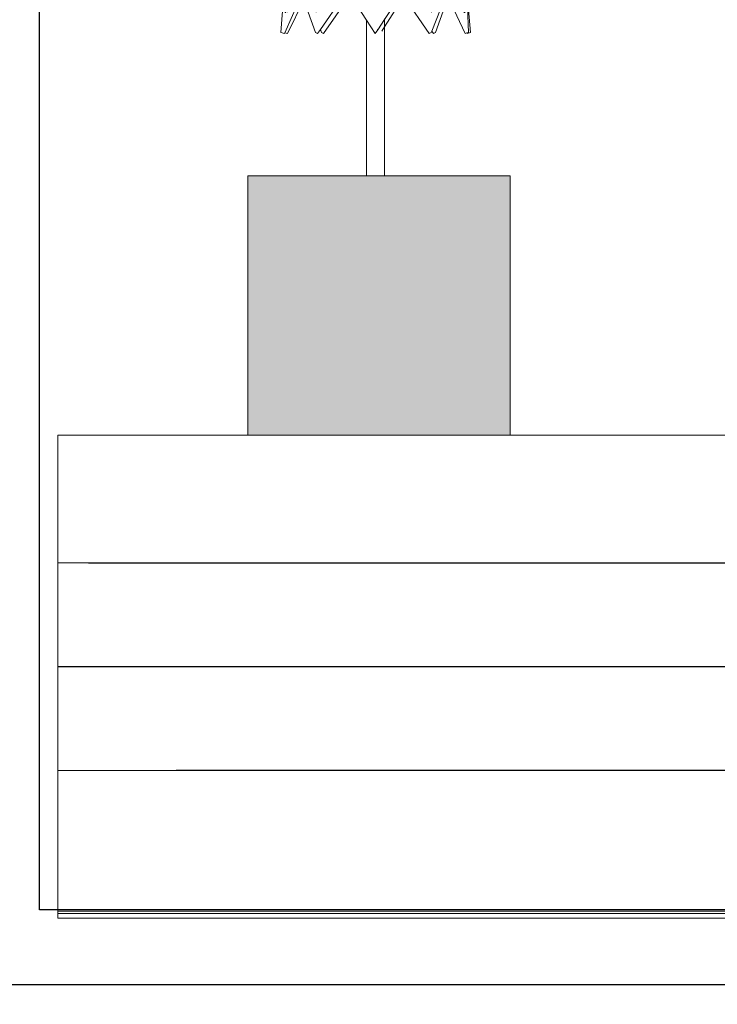
# Model space of a CAD drawing. Units: millimetres. Extents: x 7894 to 8038, y 6851 to 6951.
# Tile 3 of 49: x 7944.854 to 7949.503, y 6864.931 to 6871.489. Entities that reach past the tile are written whole.
import ezdxf

# ---------------------------------------------------------------- set-up
doc = ezdxf.new("R2010")
doc.units = ezdxf.units.MM
for name, color, linetype, lineweight in [('A-ANNO-DIMS', 2, 'Continuous', 18), ('A-FURN-ACCS', 8, 'Continuous', 13), ('A-FURN-BOOK', 8, 'Continuous', 13), ('A-FURN-CASE', 7, 'Continuous', 30)]:
    doc.layers.add(name, color=color, linetype=linetype, lineweight=lineweight)
doc.layers.add('A-FURN-ACCS-PATT', color=116, linetype='Continuous', lineweight=9, true_color=0x136734)
doc.styles.get("Standard").update_dxf_attribs({"font": 'arial.ttf'})
doc.dimstyles.new('ISO-25', dxfattribs={"dimtxt": 1, "dimasz": 1, "dimexe": 1.25, "dimexo": 0.625, "dimtad": 1, "dimdec": 0, "dimlunit": 4, "dimtxsty": 'Standard', "dimcen": 2.5, "dimclrt": 1, "dimadec": 0, "dimazin": 0, "dimtfac": 1, "dimtdec": 0, "dimtmove": 0, "dimatfit": 3, "dimfxl": 1, "dimarcsym": 0})

# ---------------------------------------------------------------- blocks, each defined once
blk = doc.blocks.new('DISPLAY-LEAF-FINIAL')
for p, q in [((2.4341, 3.4699), (2.4472, 3.4778)), ((2.4472, 3.4778), (2.4609, 3.4849)), ((2.4609, 3.4849), (2.475, 3.4911)), ((2.475, 3.4911), (2.4894, 3.4964)), ((2.4894, 3.4964), (2.5041, 3.5007)), ((2.5041, 3.5007), (2.5191, 3.5041)), ((2.5634, 3.479), (2.5605, 3.4646)), ((2.5649, 3.4937), (2.5634, 3.479)), ((2.565, 3.5085), (2.5649, 3.4937)), ((2.2094, 3.3343), (2.2756, 3.4413)), ((2.2756, 3.4413), (2.398, 3.4413)), ((2.398, 3.4413), (2.4094, 3.4516)), ((2.4094, 3.4516), (2.4214, 3.4612)), ((2.4214, 3.4612), (2.4341, 3.4699)), ((2.5358, 3.4113), (2.5266, 3.3997)), ((2.5438, 3.4237), (2.5358, 3.4113)), ((2.5507, 3.4368), (2.5438, 3.4237)), ((2.5562, 3.4504), (2.5507, 3.4368)), ((2.5605, 3.4646), (2.5562, 3.4504)), ((2.4932, 3.3709), (2.4804, 3.3635)), ((2.4804, 3.3635), (2.4804, 3.3164)), ((2.5053, 3.3794), (2.4932, 3.3709)), ((2.5164, 3.3891), (2.5053, 3.3794)), ((2.5266, 3.3997), (2.5164, 3.3891)), ((2.5489, 3.3378), (2.5584, 3.3473)), ((2.5584, 3.3473), (2.5687, 3.3558)), ((2.5687, 3.3558), (2.5799, 3.3633)), ((2.5799, 3.3633), (2.5917, 3.3696)), ((2.5917, 3.3696), (2.604, 3.3748)), ((2.604, 3.3748), (2.6168, 3.3788)), ((2.6168, 3.3788), (2.63, 3.3815)), ((2.63, 3.3815), (2.6433, 3.3829)), ((2.6433, 3.3829), (2.6567, 3.3831)), ((2.6701, 3.3819), (2.6462, 3.3254)), ((2.6567, 3.3831), (2.6701, 3.3819)), ((2.0233, 3.2209), (2.1272, 3.3343)), ((2.1272, 3.3343), (2.2094, 3.3343)), ((2.4804, 3.3164), (2.5329, 3.3164)), ((2.5329, 3.3164), (2.5404, 3.3275)), ((2.5404, 3.3275), (2.5489, 3.3378)), ((2.6462, 3.3254), (2.6199, 3.27)), ((1.7926, 3.2108), (1.8166, 3.2158)), ((1.8166, 3.2158), (1.8408, 3.2199)), ((1.8408, 3.2199), (1.8651, 3.2232)), ((1.9139, 3.2271), (1.8536, 3.1329)), ((1.8651, 3.2232), (1.8895, 3.2256)), ((1.8895, 3.2256), (1.9139, 3.2271)), ((1.934, 3.1854), (2.0233, 3.2209)), ((2.5912, 3.2159), (2.56, 3.1631)), ((2.6199, 3.27), (2.5912, 3.2159)), ((1.3282, 3.1326), (1.3879, 3.1503)), ((1.3879, 3.1503), (1.4487, 3.1639)), ((1.4487, 3.1639), (1.5102, 3.1734)), ((1.5102, 3.1734), (1.5723, 3.1786)), ((1.5723, 3.1786), (1.5113, 3.0242)), ((1.5498, 3.0242), (1.6318, 3.1522)), ((1.6318, 3.1522), (1.6538, 3.163)), ((1.6538, 3.163), (1.6762, 3.173)), ((1.6762, 3.173), (1.6989, 3.1822)), ((1.6989, 3.1822), (1.7219, 3.1906)), ((1.7219, 3.1906), (1.7453, 3.1982)), ((1.7453, 3.1982), (1.7688, 3.2049)), ((1.7688, 3.2049), (1.7926, 3.2108)), ((1.934, 3.1329), (1.934, 3.1854)), ((2.56, 3.1631), (2.5265, 3.1117)), ((1.1581, 3.0558), (1.213, 3.0852)), ((1.213, 3.0852), (1.2698, 3.1109)), ((1.2698, 3.1109), (1.3282, 3.1326)), ((1.8536, 3.1329), (1.934, 3.1329)), ((2.5265, 3.1117), (2.4908, 3.0619)), ((1.0549, 2.9861), (1.1053, 3.0227)), ((1.1053, 3.0227), (1.1581, 3.0558)), ((1.5113, 3.0242), (1.5498, 3.0242)), ((2.4908, 3.0619), (2.4529, 3.0137)), ((1.0071, 2.9462), (1.0549, 2.9861)), ((2.4129, 2.9672), (2.3708, 2.9226)), ((2.4529, 3.0137), (2.4129, 2.9672)), ((0.634, 2.9001), (0.4633, 2.6089)), ((0.6052, 2.9243), (0.5471, 2.8395)), ((0.634, 2.9046), (0.5471, 2.8395)), ((0.634, 2.9046), (0.6052, 2.9243)), ((0.634, 2.9001), (0.634, 2.9046)), ((0.6629, 2.8848), (0.634, 2.9046)), ((0.9202, 2.857), (0.9622, 2.9031)), ((0.9622, 2.9031), (1.0071, 2.9462)), ((2.3708, 2.9226), (2.3268, 2.8799)), ((0.5471, 2.8395), (0.379, 2.7129)), ((0.5989, 2.7915), (0.6629, 2.8848)), ((0.9202, 2.857), (0.8844, 2.7861)), ((1.8829, 2.8172), (1.8849, 2.8243)), ((1.8849, 2.8243), (1.8885, 2.8306)), ((1.8885, 2.8306), (1.8937, 2.8357)), ((1.8937, 2.8357), (1.9001, 2.8393)), ((1.9001, 2.8393), (1.9071, 2.8412)), ((1.9071, 2.8412), (1.9144, 2.8411)), ((1.9144, 2.8411), (1.9215, 2.8392)), ((1.9215, 2.8392), (1.9278, 2.8355)), ((1.9278, 2.8355), (1.9329, 2.8303)), ((1.9329, 2.8303), (1.9365, 2.824)), ((1.9365, 2.824), (1.9384, 2.8169)), ((2.281, 2.8392), (2.2333, 2.8006)), ((2.3268, 2.8799), (2.281, 2.8392)), ((0.5406, 2.6956), (0.5989, 2.7915)), ((0.8844, 2.7861), (0.853, 2.7132)), ((1.8829, 2.8099), (1.8829, 2.8172)), ((1.8847, 2.8029), (1.8829, 2.8099)), ((1.8884, 2.7965), (1.8847, 2.8029)), ((1.8935, 2.7913), (1.8884, 2.7965)), ((1.8998, 2.7877), (1.8935, 2.7913)), ((1.9068, 2.7857), (1.8998, 2.7877)), ((1.9141, 2.7857), (1.9068, 2.7857)), ((1.9212, 2.7875), (1.9141, 2.7857)), ((1.9275, 2.7912), (1.9212, 2.7875)), ((1.9327, 2.7963), (1.9275, 2.7912)), ((1.9364, 2.8026), (1.9327, 2.7963)), ((1.9383, 2.8096), (1.9364, 2.8026)), ((1.9384, 2.8169), (1.9383, 2.8096)), ((2.2333, 2.8006), (2.2382, 2.7921)), ((2.2382, 2.7921), (2.242, 2.7831)), ((2.242, 2.7831), (2.2446, 2.7737)), ((2.2446, 2.7737), (2.246, 2.764)), ((2.246, 2.764), (2.2462, 2.7543)), ((0.379, 2.7129), (0.2638, 2.6275)), ((0.3535, 2.675), (0.3584, 2.6897)), ((0.3584, 2.6897), (0.3671, 2.7026)), ((0.3671, 2.7026), (0.379, 2.7129)), ((0.379, 2.7129), (0.3932, 2.7199)), ((0.3932, 2.7199), (0.4088, 2.7231)), ((0.4088, 2.7231), (0.4248, 2.7223)), ((0.4248, 2.7223), (0.44, 2.7176)), ((0.44, 2.7176), (0.4533, 2.7092)), ((0.4533, 2.7092), (0.464, 2.6977)), ((0.464, 2.6977), (0.4713, 2.6839)), ((0.5406, 2.6956), (0.4875, 2.5967)), ((0.853, 2.7132), (0.8261, 2.6384)), ((1.9535, 2.6918), (1.9314, 2.6843)), ((1.9751, 2.7005), (1.9535, 2.6918)), ((1.9962, 2.7106), (1.9751, 2.7005)), ((2.0073, 2.692), (1.9896, 2.6734)), ((2.0167, 2.7218), (1.9962, 2.7106)), ((2.023, 2.7124), (2.0073, 2.692)), ((2.0364, 2.7343), (2.0167, 2.7218)), ((2.0364, 2.7343), (2.023, 2.7124)), ((2.2158, 2.6954), (2.1904, 2.6768)), ((2.2231, 2.7019), (2.2158, 2.6954)), ((2.2296, 2.7092), (2.2231, 2.7019)), ((2.2352, 2.7172), (2.2296, 2.7092)), ((2.2397, 2.7259), (2.2352, 2.7172)), ((2.243, 2.7351), (2.2397, 2.7259)), ((2.2452, 2.7446), (2.243, 2.7351)), ((2.2462, 2.7543), (2.2452, 2.7446)), ((0.2638, 2.6275), (0.2535, 2.6069)), ((0.3526, 2.6596), (0.3535, 2.675)), ((0.3527, 2.6591), (0.3526, 2.6596)), ((0.3526, 2.6569), (0.3527, 2.6591)), ((0.4713, 2.6839), (0.4746, 2.6689)), ((0.4745, 2.6667), (0.4746, 2.6689)), ((0.4745, 2.6667), (0.4746, 2.6661)), ((0.8261, 2.6384), (0.804, 2.5621)), ((1.793, 2.6675), (1.7698, 2.6695)), ((1.7698, 2.6695), (1.7755, 2.6114)), ((1.8164, 2.6669), (1.793, 2.6675)), ((1.8397, 2.6677), (1.8164, 2.6669)), ((1.863, 2.6698), (1.8397, 2.6677)), ((1.886, 2.6733), (1.863, 2.6698)), ((1.9089, 2.6781), (1.886, 2.6733)), ((1.9261, 2.6301), (1.9023, 2.6204)), ((1.9314, 2.6843), (1.9089, 2.6781)), ((1.9487, 2.6423), (1.9261, 2.6301)), ((1.97, 2.6568), (1.9487, 2.6423)), ((1.9896, 2.6734), (1.97, 2.6568)), ((2.1099, 2.6273), (2.0818, 2.6131)), ((2.1374, 2.6427), (2.1099, 2.6273)), ((2.1643, 2.6592), (2.1374, 2.6427)), ((2.1904, 2.6768), (2.1643, 2.6592)), ((0.2535, 2.6069), (0.2491, 2.5845)), ((0.2491, 2.58), (0.2491, 2.5845)), ((0.2491, 2.58), (0.2508, 2.5572)), ((0.4145, 2.6055), (0.4132, 2.6029)), ((0.4608, 2.6047), (0.4152, 2.527)), ((0.4402, 2.4957), (0.4858, 2.593)), ((0.4431, 2.613), (0.4459, 2.6117)), ((0.4509, 2.6151), (0.4489, 2.6161)), ((0.4633, 2.6089), (0.4608, 2.6047)), ((0.4858, 2.593), (0.4608, 2.6047)), ((0.4633, 2.6089), (0.4875, 2.5967)), ((0.804, 2.5621), (0.7866, 2.4847)), ((1.801, 2.6079), (1.7755, 2.6114)), ((1.8266, 2.607), (1.801, 2.6079)), ((1.8523, 2.6088), (1.8266, 2.607)), ((1.8776, 2.6133), (1.8523, 2.6088)), ((1.9023, 2.6204), (1.8776, 2.6133)), ((1.9336, 2.5606), (1.9029, 2.5538)), ((1.9641, 2.5686), (1.9336, 2.5606)), ((1.9942, 2.5779), (1.9641, 2.5686)), ((2.0239, 2.5884), (1.9942, 2.5779)), ((2.0531, 2.6002), (2.0239, 2.5884)), ((2.0818, 2.6131), (2.0531, 2.6002)), ((0.2508, 2.5572), (0.2586, 2.5356)), ((0.2586, 2.5356), (0.2719, 2.5167)), ((0.2719, 2.5167), (0.2898, 2.5018)), ((0.2898, 2.5018), (0.3111, 2.4919)), ((0.3628, 2.4909), (0.3802, 2.4968)), ((0.3649, 2.4962), (0.3628, 2.4909)), ((0.3802, 2.4968), (0.3998, 2.5097)), ((0.3978, 2.391), (0.4399, 2.495)), ((0.3983, 2.5132), (0.4016, 2.5117)), ((0.3998, 2.5097), (0.4016, 2.5117)), ((0.4029, 2.5132), (0.4004, 2.5144)), ((0.4016, 2.5117), (0.4029, 2.5132)), ((0.4016, 2.5117), (0.4399, 2.495)), ((0.4029, 2.5132), (0.4152, 2.527)), ((0.4029, 2.5132), (0.4402, 2.4957)), ((0.4085, 2.5106), (0.4078, 2.509)), ((0.4202, 2.5355), (0.4085, 2.5106)), ((1.9029, 2.5538), (1.8718, 2.5484)), ((1.8718, 2.5484), (1.8718, 2.5082)), ((1.8718, 2.5082), (1.885, 2.5088)), ((1.885, 2.5088), (1.8981, 2.5098)), ((1.8981, 2.5098), (1.9112, 2.5112)), ((1.9112, 2.5112), (1.9243, 2.513)), ((1.9243, 2.513), (1.9373, 2.5152)), ((1.9373, 2.5152), (1.9502, 2.5177)), ((1.9502, 2.5177), (1.9631, 2.5206)), ((1.9631, 2.5206), (1.9758, 2.5239)), ((1.9758, 2.5239), (1.9885, 2.5276)), ((1.9885, 2.5276), (2.001, 2.5317)), ((2.0257, 2.5409), (1.9968, 2.4843)), ((2.001, 2.5317), (2.0134, 2.5361)), ((2.0134, 2.5361), (2.0257, 2.5409)), ((0.3111, 2.4919), (0.3343, 2.4876)), ((0.3628, 2.4909), (0.3323, 2.4155)), ((0.3343, 2.4876), (0.3579, 2.4893)), ((0.3579, 2.4893), (0.3628, 2.4909)), ((0.7866, 2.4847), (0.774, 2.4062)), ((1.1928, 2.4521), (1.1631, 2.4165)), ((1.1981, 2.4572), (1.1928, 2.4521)), ((1.2041, 2.4615), (1.1981, 2.4572)), ((1.2106, 2.465), (1.2041, 2.4615)), ((1.2175, 2.4675), (1.2106, 2.465)), ((1.2247, 2.469), (1.2175, 2.4675)), ((1.2321, 2.4695), (1.2247, 2.469)), ((1.2395, 2.469), (1.2321, 2.4695)), ((1.2467, 2.4675), (1.2395, 2.469)), ((1.2536, 2.465), (1.2467, 2.4675)), ((1.2601, 2.4615), (1.2536, 2.465)), ((1.2661, 2.4572), (1.2601, 2.4615)), ((1.2714, 2.4521), (1.2661, 2.4572)), ((1.274, 2.435), (1.2714, 2.4521)), ((1.278, 2.4183), (1.274, 2.435)), ((1.9607, 2.4321), (1.918, 2.3851)), ((1.9968, 2.4843), (1.9607, 2.4321)), ((0.3323, 2.4155), (0.2946, 2.3057)), ((0.3614, 2.2848), (0.3978, 2.391)), ((0.774, 2.4062), (0.7662, 2.3272)), ((1.1364, 2.3787), (1.1127, 2.339)), ((1.1631, 2.4165), (1.1364, 2.3787)), ((1.2834, 2.4019), (1.278, 2.4183)), ((1.2903, 2.3861), (1.2834, 2.4019)), ((1.2985, 2.371), (1.2903, 2.3861)), ((1.308, 2.3566), (1.2985, 2.371)), ((1.918, 2.3851), (1.8695, 2.3441)), ((0.2946, 2.3057), (0.263, 2.1941)), ((0.7662, 2.3272), (0.7634, 2.2478)), ((1.0923, 2.2975), (1.0752, 2.2545)), ((1.1127, 2.339), (1.0923, 2.2975)), ((1.3187, 2.3431), (1.308, 2.3566)), ((1.3305, 2.3306), (1.3187, 2.3431)), ((1.3434, 2.3192), (1.3305, 2.3306)), ((1.3572, 2.3089), (1.3434, 2.3192)), ((1.3719, 2.2999), (1.3572, 2.3089)), ((1.3873, 2.2921), (1.3719, 2.2999)), ((1.8161, 2.3099), (1.7585, 2.283)), ((1.8695, 2.3441), (1.8161, 2.3099)), ((0.2147, 2.201), (0.2202, 2.2445)), ((0.223, 2.2445), (0.2147, 2.201)), ((0.223, 2.2445), (0.2202, 2.2445)), ((0.223, 2.2445), (0.2299, 2.2445)), ((0.2325, 2.2195), (0.2299, 2.2445)), ((0.3171, 2.2068), (0.3302, 2.2445)), ((0.3385, 2.2445), (0.3171, 2.2068)), ((0.3318, 2.2445), (0.3302, 2.2445)), ((0.3441, 2.2445), (0.3385, 2.2445)), ((0.3472, 2.2349), (0.3441, 2.2445)), ((0.3472, 2.2349), (0.3614, 2.2848)), ((0.3543, 2.2133), (0.3472, 2.2349)), ((0.5072, 2.2093), (0.5246, 2.2445)), ((0.5322, 2.2392), (0.5072, 2.2093)), ((0.5277, 2.2445), (0.5246, 2.2445)), ((0.5277, 2.2445), (0.5322, 2.2392)), ((0.5366, 2.2445), (0.5322, 2.2392)), ((0.5399, 2.2445), (0.5366, 2.2445)), ((0.5559, 2.2114), (0.5399, 2.2445)), ((0.7634, 2.2478), (0.7651, 2.1857)), ((0.8207, 2.2445), (0.7651, 2.1857)), ((0.93, 2.0453), (0.8207, 2.2445)), ((1.0703, 2.2388), (0.9394, 2.0859)), ((1.0703, 2.2388), (1.069, 2.2345)), ((1.0707, 2.2401), (1.0703, 2.2388)), ((1.0703, 2.2388), (1.0715, 2.2374)), ((1.0752, 2.2545), (1.0707, 2.2401)), ((1.0745, 2.2445), (1.0707, 2.2401)), ((1.0745, 2.2445), (1.0775, 2.2445)), ((1.0949, 2.2093), (1.0775, 2.2445)), ((1.2478, 2.2133), (1.2581, 2.2445)), ((1.2651, 2.2421), (1.2478, 2.2133)), ((1.2581, 2.2445), (1.2637, 2.2445)), ((1.2637, 2.2445), (1.2651, 2.2421)), ((1.2666, 2.2445), (1.2651, 2.2421)), ((1.2666, 2.2445), (1.272, 2.2445)), ((1.2851, 2.2068), (1.272, 2.2445)), ((1.3697, 2.2195), (1.3722, 2.2445)), ((1.3751, 2.2445), (1.3697, 2.2195)), ((1.3722, 2.2445), (1.3751, 2.2445)), ((1.3751, 2.2445), (1.3819, 2.2445)), ((1.3819, 2.2445), (1.3889, 2.1901)), ((1.4469, 2.2701), (1.3873, 2.2921)), ((1.5088, 2.256), (1.4469, 2.2701)), ((1.572, 2.2503), (1.5088, 2.256)), ((1.6355, 2.2529), (1.572, 2.2503)), ((1.698, 2.2639), (1.6355, 2.2529)), ((1.7585, 2.283), (1.698, 2.2639)), ((0.2133, 2.1901), (0.1946, 2.0859)), ((0.2133, 2.1901), (0.2147, 2.201)), ((0.2325, 2.2195), (0.2504, 2.1381)), ((0.2439, 2.1095), (0.2325, 2.2195)), ((0.3171, 2.2068), (0.2485, 2.0859)), ((0.263, 2.1941), (0.2504, 2.1381)), ((0.2969, 2.1855), (0.2916, 2.1618)), ((0.3543, 2.2133), (0.4197, 2.1042)), ((0.4044, 2.0607), (0.3543, 2.2133)), ((0.5072, 2.2093), (0.4197, 2.1042)), ((0.5482, 2.2204), (0.5559, 2.2114)), ((0.5559, 2.2114), (0.6628, 2.0859)), ((0.636, 2.0453), (0.5559, 2.2114)), ((0.7651, 2.1857), (0.6705, 2.0859)), ((1.0949, 2.2093), (1.1824, 2.1042)), ((1.0949, 2.2093), (1.1714, 2.0542)), ((1.2478, 2.2133), (1.1824, 2.1042)), ((1.2851, 2.2068), (1.3441, 2.1028)), ((1.2851, 2.2068), (1.3403, 2.0478)), ((1.3697, 2.2195), (1.3441, 2.1028)), ((1.3889, 2.1901), (1.4075, 2.0859)), ((1.4073, 2.0453), (1.3889, 2.1901)), ((0.2439, 2.1095), (0.2392, 2.0887)), ((0.2504, 2.1381), (0.2439, 2.1095)), ((0.2485, 2.0654), (0.2439, 2.1095)), ((0.2504, 2.1381), (0.2555, 2.1145)), ((0.4197, 2.1042), (0.4044, 2.0859)), ((1.1824, 2.1042), (1.1714, 2.0859)), ((1.3441, 2.1028), (1.3403, 2.0859)), ((0.1946, 2.0859), (0.1952, 2.0478)), ((0.1949, 2.0453), (0.1946, 1.903)), ((0.1949, 2.0453), (0.1952, 2.0478)), ((0.2485, 2.0859), (0.2485, 2.0654)), ((0.2485, 2.0654), (0.2485, 1.9035)), ((0.4044, 2.0859), (0.4044, 2.0607)), ((0.4044, 2.0607), (0.4044, 1.9015)), ((0.636, 2.0453), (0.6371, 1.9035)), ((0.6628, 2.0859), (0.6628, 1.9035)), ((0.6705, 2.0859), (0.6705, 1.9035)), ((0.93, 2.0453), (0.9309, 1.9342)), ((0.9394, 2.0859), (0.9394, 1.9343)), ((1.1714, 2.0859), (1.1714, 2.0542)), ((1.1758, 2.0453), (1.1714, 2.0542)), ((1.1758, 2.0453), (1.1768, 1.9142)), ((1.3403, 2.0859), (1.3403, 2.0478)), ((1.3412, 2.0453), (1.3403, 2.0478)), ((1.3412, 2.0453), (1.342, 1.9035)), ((1.4075, 2.0859), (1.4073, 2.0453)), ((1.4073, 2.0453), (1.4075, 1.903)), ((0.2074, 1.9648), (0.2082, 1.9727)), ((0.2082, 1.9727), (0.2095, 1.9791)), ((0.2095, 1.9791), (0.211, 1.9837)), ((0.2108, 1.9648), (0.2117, 1.9727)), ((0.211, 1.9837), (0.2126, 1.986)), ((0.2117, 1.9727), (0.2129, 1.9791)), ((0.2161, 1.986), (0.2126, 1.986)), ((0.2129, 1.9791), (0.2144, 1.9837)), ((0.2144, 1.9837), (0.2161, 1.986)), ((0.2179, 1.9725), (0.2168, 1.9646)), ((0.2194, 1.979), (0.2179, 1.9725)), ((0.2179, 1.9725), (0.218, 1.9665)), ((0.2202, 1.9812), (0.2194, 1.979)), ((0.2204, 1.9806), (0.2194, 1.979)), ((0.2213, 1.9725), (0.2202, 1.9646)), ((0.2218, 1.9746), (0.2213, 1.9725)), ((0.2969, 1.9648), (0.2997, 1.9727)), ((0.2997, 1.9727), (0.3035, 1.9791)), ((0.3035, 1.9791), (0.3083, 1.9837)), ((0.3083, 1.9837), (0.3136, 1.986)), ((0.3164, 1.986), (0.3136, 1.986)), ((0.478, 1.9648), (0.482, 1.9727)), ((0.482, 1.9727), (0.4877, 1.9791)), ((0.4877, 1.9791), (0.4947, 1.9837)), ((0.4947, 1.9837), (0.5025, 1.986)), ((0.5041, 1.986), (0.5025, 1.986)), ((0.756, 1.9648), (0.7606, 1.9727)), ((0.7606, 1.9727), (0.7671, 1.9791)), ((0.7671, 1.9791), (0.775, 1.9837)), ((0.775, 1.9837), (0.7838, 1.986)), ((0.7838, 1.986), (0.793, 1.986)), ((0.793, 1.986), (0.8018, 1.9836)), ((0.8018, 1.9836), (0.8096, 1.979)), ((0.8096, 1.979), (0.8161, 1.9725)), ((0.8161, 1.9725), (0.8206, 1.9646)), ((1.0443, 1.986), (1.0459, 1.986)), ((1.0459, 1.986), (1.0541, 1.986)), ((1.0541, 1.986), (1.062, 1.9836)), ((1.062, 1.9836), (1.0691, 1.979)), ((1.0691, 1.979), (1.0749, 1.9725)), ((1.0749, 1.9725), (1.079, 1.9646)), ((1.2486, 1.986), (1.2513, 1.986)), ((1.2513, 1.986), (1.2571, 1.986)), ((1.2571, 1.986), (1.2627, 1.9836)), ((1.2627, 1.9836), (1.2677, 1.979)), ((1.2677, 1.979), (1.2717, 1.9725)), ((1.2717, 1.9725), (1.2746, 1.9646)), ((1.3734, 1.986), (1.3755, 1.986)), ((1.3755, 1.986), (1.3775, 1.9836)), ((1.3755, 1.986), (1.3768, 1.986)), ((1.3768, 1.986), (1.3789, 1.986)), ((1.3775, 1.9836), (1.3794, 1.979)), ((1.3789, 1.986), (1.3809, 1.9836)), ((1.3794, 1.979), (1.3809, 1.9725)), ((1.3809, 1.9836), (1.3828, 1.979)), ((1.3809, 1.9725), (1.3819, 1.9646)), ((1.3828, 1.979), (1.3843, 1.9725)), ((1.3843, 1.9725), (1.3853, 1.9646)), ((0.1887, 1.9015), (0.1946, 1.903)), ((0.1946, 1.903), (0.1964, 1.9035)), ((0.1946, 1.903), (0.1946, 1.9015)), ((0.1964, 1.9035), (0.1977, 1.9034)), ((0.1964, 1.9035), (0.1969, 1.9035)), ((0.2373, 1.9035), (0.1977, 1.9034)), ((0.2069, 1.956), (0.2074, 1.9648)), ((0.2069, 1.9469), (0.2069, 1.956)), ((0.2074, 1.938), (0.2069, 1.9469)), ((0.2082, 1.9301), (0.2074, 1.938)), ((0.2094, 1.9236), (0.2082, 1.9301)), ((0.2109, 1.9191), (0.2094, 1.9236)), ((0.2103, 1.9469), (0.2104, 1.956)), ((0.2108, 1.938), (0.2103, 1.9469)), ((0.2104, 1.956), (0.2108, 1.9648)), ((0.2116, 1.9301), (0.2108, 1.938)), ((0.2126, 1.9167), (0.2109, 1.9191)), ((0.2129, 1.9236), (0.2116, 1.9301)), ((0.2143, 1.9167), (0.2126, 1.9167)), ((0.2163, 1.9467), (0.2129, 1.9236)), ((0.2144, 1.9191), (0.2129, 1.9236)), ((0.216, 1.9167), (0.2143, 1.9167)), ((0.216, 1.9167), (0.2144, 1.9191)), ((0.2177, 1.9167), (0.216, 1.9167)), ((0.2168, 1.9646), (0.2163, 1.9558)), ((0.2163, 1.9558), (0.2163, 1.9467)), ((0.2163, 1.9467), (0.2168, 1.9379)), ((0.218, 1.9665), (0.2168, 1.9646)), ((0.2168, 1.9379), (0.2179, 1.93)), ((0.2179, 1.93), (0.2194, 1.9235)), ((0.2194, 1.9235), (0.2202, 1.9215)), ((0.2202, 1.9646), (0.2197, 1.9558)), ((0.2197, 1.9558), (0.2197, 1.9467)), ((0.2197, 1.9467), (0.2202, 1.9379)), ((0.2202, 1.9379), (0.2213, 1.93)), ((0.2213, 1.93), (0.2218, 1.928)), ((0.2485, 1.9035), (0.2439, 1.9035)), ((0.2485, 1.9251), (0.2458, 1.9015)), ((0.2485, 1.9035), (0.2485, 1.9015)), ((0.3913, 1.9035), (0.265, 1.9035)), ((0.2955, 1.956), (0.2969, 1.9648)), ((0.2955, 1.9469), (0.2955, 1.956)), ((0.2969, 1.938), (0.2955, 1.9469)), ((0.2996, 1.9301), (0.2969, 1.938)), ((0.3034, 1.9236), (0.2996, 1.9301)), ((0.3082, 1.9191), (0.3034, 1.9236)), ((0.3134, 1.9167), (0.3082, 1.9191)), ((0.3189, 1.9167), (0.3134, 1.9167)), ((0.3217, 1.9167), (0.3189, 1.9167)), ((0.4385, 1.9035), (0.6066, 1.9035)), ((0.4759, 1.956), (0.478, 1.9648)), ((0.4759, 1.9469), (0.4759, 1.956)), ((0.478, 1.938), (0.4759, 1.9469)), ((0.4819, 1.9301), (0.478, 1.938)), ((0.4876, 1.9236), (0.4819, 1.9301)), ((0.4945, 1.9191), (0.4876, 1.9236)), ((0.5023, 1.9167), (0.4945, 1.9191)), ((0.5103, 1.9167), (0.5023, 1.9167)), ((0.512, 1.9167), (0.5103, 1.9167)), ((0.6371, 1.9035), (0.6338, 1.9035)), ((0.6371, 1.9035), (0.6371, 1.9015)), ((0.6628, 1.9035), (0.6371, 1.9035)), ((0.6628, 1.9035), (0.6705, 1.9035)), ((0.6628, 1.9035), (0.6628, 1.9015)), ((0.6705, 1.9035), (0.6705, 1.9015)), ((0.7081, 1.9035), (0.894, 1.9035)), ((0.7536, 1.9469), (0.7537, 1.956)), ((0.756, 1.938), (0.7536, 1.9469)), ((0.7537, 1.956), (0.756, 1.9648)), ((0.7605, 1.9301), (0.756, 1.938)), ((0.7669, 1.9236), (0.7605, 1.9301)), ((0.7748, 1.9191), (0.7669, 1.9236)), ((0.7836, 1.9167), (0.7748, 1.9191)), ((0.7928, 1.9167), (0.7836, 1.9167)), ((0.8016, 1.919), (0.7928, 1.9167)), ((0.8095, 1.9235), (0.8016, 1.919)), ((0.816, 1.93), (0.8095, 1.9235)), ((0.8206, 1.9379), (0.816, 1.93)), ((0.8206, 1.9646), (0.823, 1.9558)), ((0.8229, 1.9467), (0.8206, 1.9379)), ((0.823, 1.9558), (0.8229, 1.9467)), ((0.9394, 1.9343), (0.9309, 1.9342)), ((0.9309, 1.9342), (0.9312, 1.9035)), ((0.9312, 1.9035), (0.9312, 1.9015)), ((0.9394, 1.9035), (0.9312, 1.9035)), ((0.9424, 1.9343), (0.9394, 1.9343)), ((0.9394, 1.9343), (0.9394, 1.9035)), ((0.9424, 1.9035), (0.9394, 1.9035)), ((0.9394, 1.9035), (0.9394, 1.9015)), ((0.9534, 1.9035), (1.1456, 1.9035)), ((1.0224, 1.935), (1.0209, 1.935)), ((1.0524, 1.9167), (1.0539, 1.9167)), ((1.0618, 1.919), (1.0539, 1.9167)), ((1.069, 1.9235), (1.0618, 1.919)), ((1.0748, 1.93), (1.069, 1.9235)), ((1.0789, 1.9379), (1.0748, 1.93)), ((1.0811, 1.9467), (1.0789, 1.9379)), ((1.079, 1.9646), (1.0811, 1.9558)), ((1.0811, 1.9558), (1.0811, 1.9467)), ((1.3304, 1.9035), (1.1965, 1.9035)), ((1.2543, 1.9167), (1.257, 1.9167)), ((1.2626, 1.919), (1.257, 1.9167)), ((1.2676, 1.9235), (1.2626, 1.919)), ((1.2717, 1.93), (1.2676, 1.9235)), ((1.2746, 1.9379), (1.2717, 1.93)), ((1.2746, 1.9646), (1.2761, 1.9558)), ((1.2761, 1.9467), (1.2746, 1.9379)), ((1.2761, 1.9558), (1.2761, 1.9467)), ((1.3471, 1.9035), (1.342, 1.9035)), ((1.342, 1.9035), (1.342, 1.9015)), ((1.3561, 1.9035), (1.4004, 1.9035)), ((1.3775, 1.919), (1.3755, 1.9167)), ((1.3755, 1.9167), (1.3789, 1.9167)), ((1.3793, 1.9235), (1.3775, 1.919)), ((1.3809, 1.919), (1.3789, 1.9167)), ((1.3808, 1.93), (1.3793, 1.9235)), ((1.3819, 1.9379), (1.3808, 1.93)), ((1.3827, 1.9235), (1.3809, 1.919)), ((1.3819, 1.9646), (1.3825, 1.9558)), ((1.3825, 1.9467), (1.3819, 1.9379)), ((1.3825, 1.9558), (1.3825, 1.9467)), ((1.3842, 1.93), (1.3827, 1.9235)), ((1.3853, 1.9379), (1.3842, 1.93)), ((1.3853, 1.9646), (1.3859, 1.9558)), ((1.3859, 1.9467), (1.3853, 1.9379)), ((1.3859, 1.9558), (1.3859, 1.9467)), ((1.4075, 1.903), (1.4135, 1.9015)), ((1.4075, 1.903), (1.4075, 1.9015)), ((0, 1.6201), (0.181, 1.8491)), ((0.1696, 1.8695), (0.1697, 1.8775)), ((0.1715, 1.8618), (0.1696, 1.8695)), ((0.1697, 1.8775), (0.1719, 1.8852)), ((0.1754, 1.8548), (0.1715, 1.8618)), ((0.1719, 1.8852), (0.176, 1.892)), ((0.181, 1.8491), (0.1754, 1.8548)), ((0.176, 1.892), (0.1817, 1.8976)), ((0.1817, 1.8976), (0.1887, 1.9015)), ((0.1946, 1.8976), (0.1945, 1.8695)), ((0.1945, 1.8618), (0.1945, 1.8548)), ((0.1952, 1.8548), (0.1945, 1.8548)), ((0.2052, 1.8548), (0.1945, 1.8548)), ((0.2048, 1.8513), (0.2047, 1.8491)), ((0.2052, 1.8548), (0.2048, 1.8513)), ((0.2485, 1.8548), (0.2052, 1.8548)), ((0.2404, 1.8548), (0.2398, 1.8491)), ((0.2485, 1.8971), (0.2439, 1.8971)), ((0.2453, 1.8976), (0.244, 1.8856)), ((0.2485, 1.8976), (0.2485, 1.8971)), ((0.2485, 1.8971), (0.2485, 1.8695)), ((0.2485, 1.8618), (0.2485, 1.8548)), ((0.2485, 1.8548), (0.2756, 1.8548)), ((0.275, 1.8491), (0.2756, 1.8548)), ((0.2756, 1.8548), (0.4049, 1.8548)), ((0.4044, 1.8976), (0.4044, 1.8695)), ((0.4044, 1.8618), (0.4049, 1.8548)), ((0.4049, 1.8548), (0.6375, 1.8548)), ((0.6371, 1.8971), (0.6338, 1.8971)), ((0.6371, 1.8976), (0.6371, 1.8971)), ((0.6371, 1.8971), (0.6374, 1.8695)), ((0.6628, 1.8971), (0.6371, 1.8971)), ((0.6374, 1.8618), (0.6375, 1.8548)), ((0.6628, 1.8548), (0.6375, 1.8548)), ((0.6628, 1.8976), (0.6628, 1.8971)), ((0.6628, 1.8971), (0.6628, 1.8695)), ((0.6705, 1.8971), (0.6628, 1.8971)), ((0.6628, 1.8618), (0.6628, 1.8548)), ((0.6705, 1.8976), (0.6705, 1.8971)), ((0.6705, 1.8971), (0.6705, 1.8695)), ((0.6705, 1.8618), (0.6705, 1.8548)), ((0.6705, 1.8548), (0.9316, 1.8548)), ((0.9313, 1.8976), (0.9313, 1.8971)), ((0.9313, 1.8971), (0.9315, 1.8695)), ((0.9394, 1.8971), (0.9313, 1.8971)), ((0.9316, 1.8618), (0.9316, 1.8548)), ((0.9394, 1.8548), (0.9316, 1.8548)), ((0.9394, 1.8976), (0.9394, 1.8971)), ((0.9424, 1.8971), (0.9394, 1.8971)), ((0.9394, 1.8971), (0.9394, 1.8695)), ((0.9394, 1.8618), (0.9394, 1.8548)), ((1.3422, 1.8548), (0.9394, 1.8548)), ((1.342, 1.8976), (1.342, 1.8971)), ((1.3471, 1.8971), (1.342, 1.8971)), ((1.342, 1.8971), (1.3421, 1.8695)), ((1.3422, 1.8618), (1.3422, 1.8548)), ((1.4075, 1.8548), (1.3422, 1.8548)), ((1.4075, 1.8976), (1.4075, 1.8695)), ((1.4075, 1.8618), (1.4075, 1.8548)), ((1.4135, 1.9015), (1.4205, 1.8976)), ((1.4205, 1.8976), (1.4262, 1.892)), ((1.4267, 1.8548), (1.4212, 1.8491)), ((1.4212, 1.8491), (1.6021, 1.6201)), ((1.4262, 1.892), (1.4303, 1.8852)), ((1.4306, 1.8618), (1.4267, 1.8548)), ((1.4303, 1.8852), (1.4325, 1.8775)), ((1.4326, 1.8695), (1.4306, 1.8618)), ((1.4325, 1.8775), (1.4326, 1.8695)), ((0.2072, 1.3429), (0, 1.6201)), ((1.6021, 1.6201), (0, 1.6201)), ((1.6021, 1.6201), (1.395, 1.3429)), ((0.1678, 1.3095), (0.1742, 1.3213)), ((0.1742, 1.3213), (0.1833, 1.3311)), ((0.1833, 1.3311), (0.1945, 1.3384)), ((0.1945, 1.3384), (0.2072, 1.3429)), ((1.395, 1.3429), (1.4076, 1.3384)), ((1.4076, 1.3384), (1.4188, 1.3311)), ((1.4188, 1.3311), (1.4279, 1.3213)), ((1.4279, 1.3213), (1.4344, 1.3095)), ((0.1641, 1.2831), (0.1643, 1.2966)), ((0.1672, 1.2701), (0.1641, 1.2831)), ((0.1643, 1.2966), (0.1678, 1.3095)), ((0.1733, 1.2582), (0.1672, 1.2701)), ((0.1821, 1.2481), (0.1733, 1.2582)), ((0.1931, 1.2404), (0.1821, 1.2481)), ((1.42, 1.2481), (1.4091, 1.2404)), ((1.4288, 1.2582), (1.42, 1.2481)), ((1.435, 1.2701), (1.4288, 1.2582)), ((1.4344, 1.3095), (1.4378, 1.2966)), ((1.438, 1.2831), (1.435, 1.2701)), ((1.4378, 1.2966), (1.438, 1.2831)), ((0.1714, 0.9553), (0.1907, 1.234)), ((0.2189, 1.234), (0.1907, 1.234)), ((0.2056, 1.2356), (0.1931, 1.2404)), ((0.1964, 0.9543), (0.3109, 1.2098)), ((0.2189, 1.234), (0.2056, 1.2356)), ((0.2118, 1.177), (0.2173, 1.1867)), ((0.2173, 1.1867), (0.2227, 1.1934)), ((0.2189, 1.234), (0.2969, 1.234)), ((0.2227, 1.1934), (0.2276, 1.1967)), ((0.2276, 1.1967), (0.2317, 1.1963)), ((0.2325, 1.1953), (0.2317, 1.1963)), ((0.2325, 1.1953), (0.2366, 1.1949)), ((0.2969, 1.234), (0.3023, 1.234)), ((0.3029, 1.2321), (0.2969, 1.234)), ((0.3029, 1.2321), (0.3023, 1.234)), ((0.3023, 1.234), (0.5943, 1.234)), ((0.3109, 1.2098), (0.3029, 1.2321)), ((0.3244, 1.1717), (0.3109, 1.2098)), ((0.4028, 1.177), (0.4128, 1.1867)), ((0.4128, 1.1867), (0.4241, 1.1934)), ((0.4241, 1.1934), (0.436, 1.1967)), ((0.434, 0.9751), (0.6087, 1.2276)), ((0.436, 1.1967), (0.4475, 1.1963)), ((0.4475, 1.1963), (0.4584, 1.1919)), ((0.455, 0.949), (0.6322, 1.205)), ((0.4584, 1.1919), (0.4611, 1.1909)), ((0.5943, 1.234), (0.6175, 1.234)), ((0.6087, 1.2276), (0.5943, 1.234)), ((0.6175, 1.2276), (0.6175, 1.234)), ((0.9517, 1.234), (0.6175, 1.234)), ((0.6322, 1.205), (0.6175, 1.2276)), ((0.7416, 1.0372), (0.6322, 1.205)), ((0.7597, 1.177), (0.7703, 1.1867)), ((0.7703, 1.1867), (0.7831, 1.1934)), ((0.7831, 1.1934), (0.7973, 1.1967)), ((0.7973, 1.1967), (0.8119, 1.1963)), ((0.8119, 1.1963), (0.8259, 1.1923)), ((0.8259, 1.1923), (0.8383, 1.1849)), ((0.8383, 1.1849), (0.8484, 1.1746)), ((0.8605, 1.0411), (0.9765, 1.2154)), ((0.8605, 0.9923), (0.9902, 1.1955)), ((0.9809, 1.2337), (0.9517, 1.234)), ((0.9765, 1.2154), (0.9744, 1.2185)), ((0.9902, 1.1955), (0.9765, 1.2154)), ((0.9809, 1.2337), (0.9815, 1.234)), ((0.9815, 1.234), (0.983, 1.234)), ((1.2836, 1.234), (0.983, 1.234)), ((1.16, 0.949), (0.9902, 1.1955)), ((1.1241, 1.1921), (1.1257, 1.1925)), ((1.1257, 1.1925), (1.127, 1.1934)), ((1.127, 1.1934), (1.1382, 1.1967)), ((1.1382, 1.1967), (1.1502, 1.1963)), ((1.1502, 1.1963), (1.1624, 1.1923)), ((1.1624, 1.1923), (1.1737, 1.1849)), ((1.1737, 1.1849), (1.1835, 1.1746)), ((1.1768, 0.964), (1.2748, 1.2121)), ((1.2015, 0.9553), (1.285, 1.1903)), ((1.2748, 1.2121), (1.2826, 1.2319)), ((1.285, 1.1903), (1.2748, 1.2121)), ((1.2826, 1.2319), (1.2898, 1.234)), ((1.2826, 1.2319), (1.2836, 1.234)), ((1.2836, 1.234), (1.2898, 1.234)), ((1.398, 0.949), (1.285, 1.1903)), ((1.2898, 1.234), (1.3832, 1.234)), ((1.359, 1.1953), (1.3638, 1.1967)), ((1.359, 1.1953), (1.3619, 1.1951)), ((1.3638, 1.1967), (1.3687, 1.1963)), ((1.3687, 1.1963), (1.3744, 1.1923)), ((1.3744, 1.1923), (1.3804, 1.1849)), ((1.3804, 1.1849), (1.3863, 1.1746)), ((1.3965, 1.2356), (1.3832, 1.234)), ((1.41, 1.2337), (1.3832, 1.234)), ((1.4091, 1.2404), (1.3965, 1.2356)), ((1.4111, 1.234), (1.41, 1.2337)), ((1.4113, 1.2316), (1.4111, 1.234)), ((1.4348, 0.9553), (1.4113, 1.2316)), ((1.4203, 0.9553), (1.4113, 1.2316)), ((0.1943, 1.1113), (0.1955, 1.1237)), ((0.1955, 1.1237), (0.1981, 1.1374)), ((0.1981, 1.1374), (0.2018, 1.1515)), ((0.2018, 1.1515), (0.2065, 1.165)), ((0.2065, 1.165), (0.2118, 1.177)), ((0.2147, 0.949), (0.3244, 1.1717)), ((0.4015, 0.9553), (0.3244, 1.1717)), ((0.3867, 1.1374), (0.3893, 1.1515)), ((0.3871, 1.1237), (0.3867, 1.1374)), ((0.3906, 1.1113), (0.3871, 1.1237)), ((0.3893, 1.1515), (0.3948, 1.165)), ((0.3948, 1.165), (0.4028, 1.177)), ((0.7474, 1.1361), (0.7475, 1.1373)), ((0.7475, 1.1373), (0.7478, 1.1515)), ((0.7478, 1.1515), (0.752, 1.165)), ((0.752, 1.165), (0.7597, 1.177)), ((0.8484, 1.1746), (0.8553, 1.1622)), ((0.8553, 1.1622), (0.8587, 1.1485)), ((0.8587, 1.1471), (0.8587, 1.1485)), ((1.1835, 1.1746), (1.1911, 1.1622)), ((1.1911, 1.1622), (1.196, 1.1485)), ((1.1964, 1.1209), (1.192, 1.1089)), ((1.196, 1.1485), (1.1978, 1.1344)), ((1.1978, 1.1344), (1.1964, 1.1209)), ((1.3863, 1.1746), (1.3917, 1.1622)), ((1.3917, 1.1622), (1.3963, 1.1485)), ((1.3963, 1.1485), (1.3997, 1.1344)), ((1.3997, 1.1344), (1.4018, 1.1209)), ((1.4018, 1.1209), (1.4023, 1.1089)), ((0.1946, 1.101), (0.1943, 1.1113)), ((0.1963, 1.0936), (0.1946, 1.101)), ((0.1993, 1.0896), (0.1963, 1.0936)), ((0.2034, 1.0892), (0.1993, 1.0896)), ((0.2041, 1.0883), (0.2034, 1.0892)), ((0.2112, 1.0961), (0.2129, 1.0925)), ((0.2129, 1.0925), (0.2137, 1.0919)), ((0.2141, 1.1), (0.2145, 1.0978)), ((0.3969, 1.101), (0.3906, 1.1113)), ((0.4056, 1.0936), (0.3969, 1.101)), ((0.4087, 1.0923), (0.4056, 1.0936)), ((1.1736, 1.092), (1.1723, 1.0911)), ((1.1736, 1.092), (1.1752, 1.0925)), ((1.1847, 1.0992), (1.1752, 1.0925)), ((1.192, 1.1089), (1.1847, 1.0992)), ((1.3919, 1.0894), (1.39, 1.0879)), ((1.39, 1.0879), (1.3948, 1.0892)), ((1.3987, 1.0925), (1.3948, 1.0892)), ((1.4012, 1.0992), (1.3987, 1.0925)), ((1.4023, 1.1089), (1.4012, 1.0992)), ((0.7416, 0), (0.7416, 1.0372)), ((0.7992, 0.949), (0.7416, 1.0372)), ((0.8158, 0.974), (0.8605, 1.0411)), ((0.8431, 0.9651), (0.8605, 0.9923)), ((0.8605, 1.0411), (0.8605, 1.0475)), ((0.8605, 0.9923), (0.8605, 1.0411)), ((0.8605, 0), (0.8605, 0.9923)), ((0.1941, 0.949), (0.1714, 0.9553)), ((0.1941, 0.949), (0.1964, 0.9543)), ((0.2147, 0.949), (0.1964, 0.9543)), ((0.4159, 0.949), (0.4015, 0.9553)), ((0.4159, 0.949), (0.434, 0.9751)), ((0.4421, 0.9553), (0.434, 0.9751)), ((0.455, 0.949), (0.4421, 0.9553)), ((0.7992, 0.949), (0.8158, 0.974)), ((0.8158, 0.974), (0.8137, 0.9772)), ((0.8165, 0.9731), (0.8158, 0.974)), ((1.16, 0.949), (1.1734, 0.9553)), ((1.1734, 0.9553), (1.1768, 0.964)), ((1.1872, 0.949), (1.1768, 0.964)), ((1.1872, 0.949), (1.2015, 0.9553)), ((1.398, 0.949), (1.4105, 0.9525)), ((1.4105, 0.9525), (1.4203, 0.9553)), ((1.412, 0.949), (1.4105, 0.9525)), ((1.412, 0.949), (1.4348, 0.9553))]:
    blk.add_line(p, q)
blk = doc.blocks.new('*D36')
at = {"layer": 'A-ANNO-DIMS', "color": 0, "lineweight": -2, "transparency": 16777216}
for p, q in [((7980.8359, 6877.9586), (7980.8359, 6858.5122)), ((7944.4866, 6864.4359), (7944.4866, 6858.5122)), ((7945.4866, 6859.7622), (7979.8359, 6859.7622))]:
    blk.add_line(p, q, dxfattribs=at)
at = {"layer": 'A-ANNO-DIMS', "color": 0, "transparency": 16777216}
for points in [[(7945.4866, 6859.9288), (7945.4866, 6859.5955), (7944.4866, 6859.7622)], [(7979.8359, 6859.9288), (7979.8359, 6859.5955), (7980.8359, 6859.7622)]]:
    blk.add_solid(points, dxfattribs=at)
at = {"layer": 'Defpoints', "color": 0, "transparency": 16777216}
for p in [(7980.8359, 6878.5836), (7944.4866, 6865.0609), (7980.8359, 6859.7622)]:
    blk.add_point(p, dxfattribs=at)
at = {"layer": 'A-ANNO-DIMS', "color": 1, "transparency": 16777216, "insert": (7962.6613, 6860.9046), "char_height": 1, "attachment_point": 5}
blk.add_mtext('3\'-0 1/2"', dxfattribs=at)
blk = doc.blocks.new('*D37')
at = {"layer": 'A-ANNO-DIMS', "color": 0, "lineweight": -2, "transparency": 16777216}
for p, q in [((7954.9197, 6887.9028), (7941.3891, 6887.9028)), ((7942.6391, 6862.6097), (7942.6391, 6886.9028)), ((7953.6228, 6861.6097), (7941.3891, 6861.6097))]:
    blk.add_line(p, q, dxfattribs=at)
at = {"layer": 'A-ANNO-DIMS', "color": 0, "transparency": 16777216}
for points in [[(7942.4724, 6886.9028), (7942.8057, 6886.9028), (7942.6391, 6887.9028)], [(7942.4724, 6862.6097), (7942.8057, 6862.6097), (7942.6391, 6861.6097)]]:
    blk.add_solid(points, dxfattribs=at)
at = {"layer": 'Defpoints', "color": 0, "transparency": 16777216}
for p in [(7942.6391, 6887.9028), (7955.5447, 6887.9028), (7954.2478, 6861.6097)]:
    blk.add_point(p, dxfattribs=at)
at = {"layer": 'A-ANNO-DIMS', "color": 1, "transparency": 16777216, "insert": (7941.497, 6874.7562), "char_height": 1, "attachment_point": 5, "rotation": 90}
blk.add_mtext('2\'-2 1/2"', dxfattribs=at)

msp = doc.modelspace()

# ---------------------------------------------------------------- hatches: boundary and pattern name
at = {"layer": 'A-FURN-ACCS-PATT'}
h = msp.add_hatch(color=256, dxfattribs=at)
h.dxf.hatch_style = 1
h.paths.add_polyline_path([(7948.1227, 6870.4483), (7947.284, 6870.4483), (7947.1651, 6870.4483), (7946.3749, 6870.4483), (7946.3749, 6868.7211), (7948.1227, 6868.7211)])

# ---------------------------------------------------------------- linework, layer by layer
at = {"layer": 'A-FURN-ACCS'}
for p, q in [((7946.3749, 6868.7211), (7946.3749, 6870.4483)), ((7946.3749, 6870.4483), (7947.1651, 6870.4483)), ((7947.284, 6870.4483), (7947.1651, 6870.4483)), ((7947.284, 6870.4483), (7948.1227, 6870.4483)), ((7948.1227, 6868.7211), (7948.1227, 6870.4483))]:
    msp.add_line(p, q, dxfattribs=at)
at = {"layer": 'A-FURN-BOOK'}
for p, q in [((7953.7957, 6868.7211), (7945.1072, 6868.7211)), ((7945.1072, 6865.5049), (7945.1072, 6868.7211)), ((7953.7957, 6867.871), (7945.1072, 6867.871)), ((7954.0211, 6867.8683), (7945.3118, 6867.8683)), ((7954.0211, 6867.1816), (7945.1072, 6867.1816)), ((7945.1072, 6867.1782), (7954.0292, 6867.1782)), ((7945.1072, 6866.4885), (7953.8124, 6866.4885)), ((7954.0365, 6866.4915), (7945.8962, 6866.4915)), ((7953.7178, 6865.5609), (7945.1072, 6865.5609)), ((7953.7178, 6865.5527), (7945.1072, 6865.5519)), ((7953.8102, 6865.5367), (7945.1072, 6865.5367)), ((7953.8124, 6865.5049), (7945.1072, 6865.5049))]:
    msp.add_line(p, q, dxfattribs=at)
at = {"layer": 'A-FURN-CASE'}
for points in [[(7944.4866, 6876.4609), (7955.8866, 6876.4609), (7955.8866, 6865.0609), (7944.4866, 6865.0609)], [(7944.9866, 6875.9609), (7955.3866, 6875.9609), (7955.3866, 6865.5609), (7944.9866, 6865.5609)]]:
    msp.add_lwpolyline(points, close=True, dxfattribs=at)

# ---------------------------------------------------------------- block references
at = {"layer": 'A-FURN-ACCS'}
msp.add_blockref('DISPLAY-LEAF-FINIAL', (7946.4235, 6870.4483), dxfattribs=at)

# ---------------------------------------------------------------- dimensions: what is measured, and where the dimension line sits
at = {"layer": 'A-ANNO-DIMS'}
dim = msp.add_linear_dim(base=(7942.6391, 6887.9028), p1=(7954.2478, 6861.6097), p2=(7955.5447, 6887.9028), angle=90, dimstyle='ISO-25', override={"dimdec": 1, "dimlfac": 1, "dimrnd": 0, "dimzin": 1, "dimdsep": 46, "dimlunit": 4, "dimfrac": 2}, dxfattribs=at)
dim.commit()
dim.dimension.update_dxf_attribs({"geometry": '*D37', "text_midpoint": (7941.497, 6874.7562)})
dim = msp.add_linear_dim(base=(7980.8359, 6859.7622), p1=(7944.4866, 6865.0609), p2=(7980.8359, 6878.5836), dimstyle='ISO-25', override={"dimdec": 1, "dimlfac": 1, "dimrnd": 0, "dimzin": 1, "dimdsep": 46, "dimlunit": 4, "dimfrac": 2}, dxfattribs=at)
dim.commit()
dim.dimension.update_dxf_attribs({"geometry": '*D36', "text_midpoint": (7962.6613, 6860.9046)})

doc.saveas('drawing.dxf')
